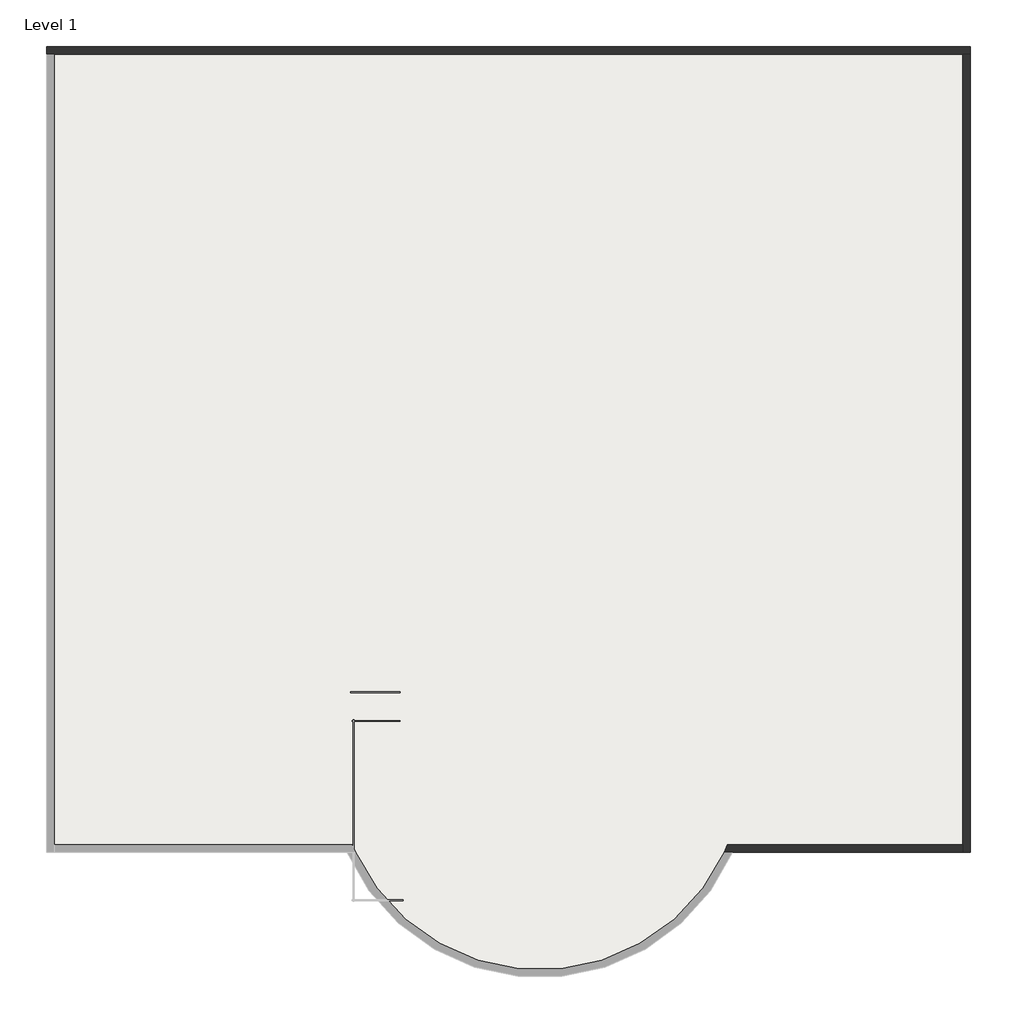
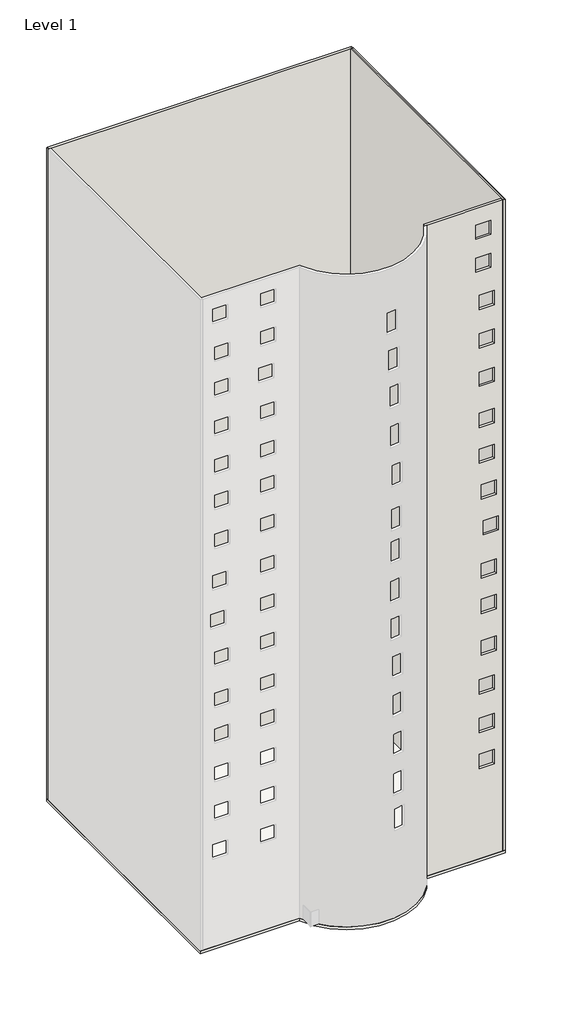
# One storey, part 3 of 3: 3 walls, 1 slab.
"""IFC4 building model written with IfcOpenShell, lengths in millimetres."""

from ifc_helpers import new_model, si_unit, point, frame, frame_2d, origin, place, context, project, spatial, polyline, circle_curve, trimmed, segment, composite_curve, outline, extrude, faceted_brep, element, save
from ifc_brep_helpers import plane_surface, revolved_surface, advanced_brep

model = new_model("IFC4")

# Units and contexts
model_context = context("Model", 3, world=origin())
ifc_project = project(units=[si_unit("LENGTHUNIT", "METRE", prefix="MILLI")], contexts=[model_context])

# Site, building, storey
site = spatial("IfcSite", under=ifc_project)
building = spatial("IfcBuilding", under=site)
storey = spatial("IfcBuildingStorey", under=building, Name="Level 1", Elevation=0.0)

# Slab
placement = place(None, origin())
element("IfcSlab", 1, ObjectType="9\"", at=placement, inside=storey, context=model_context, shape_type="SweptSolid", body=[
    extrude(outline(composite_curve([segment(polyline([(7979.2494573, 7359.5191779), (7979.2494573, -14078.0808221), (1652.8739931, -14078.0808221)]), True, "CONTINUOUS"), segment(trimmed(circle_curve(frame_2d((-3476.1505427, -11788.3650223)), 5616.9111737), [point((1652.8739931, -14078.0808221))], [point((-8605.1750786, -14078.0808221))], False, "CARTESIAN"), True, "CONTINUOUS"), segment(polyline([(-8605.1750786, -14078.0808221), (-16607.9505427, -14078.0808221), (-16607.9505427, 7359.5191779), (7979.2494573, 7359.5191779)]), True, "CONTINUOUS")], self_intersect=False)), frame((0.0, 0.0, -228.6), z_axis=(0.0, 0.0, 1.0), x_axis=(1.0, 0.0, 0.0)), (0.0, 0.0, 1.0), 228.6),
])

# Walls
element("IfcWall", 2, ObjectType="Generic - 8\"", at=placement, inside=storey, context=model_context, shape_type="Brep", body=[
    faceted_brep([(-16607.9505427, 7156.3191779, 0.0), (-16404.7505427, 7156.3191779, 0.0), (7776.0494573, 7156.3191779, 0.0), (7979.2494573, 7156.3191779, 0.0), (7979.2494573, 7156.3191779, 55473.6), (7928.4494573, 7156.3191779, 55473.6), (7776.0494573, 7156.3191779, 55473.6), (-16404.7505427, 7156.3191779, 55473.6), (-16556.2150607, 7156.3191779, 55473.6), (-16607.9505427, 7156.3191779, 55473.6), (-16607.9505427, 7359.5191779, 0.0), (-16607.9505427, 7359.5191779, 55473.6), (-16556.2150607, 7359.5191779, 55473.6), (7928.4494573, 7359.5191779, 55473.6), (7979.2494573, 7359.5191779, 55473.6), (7979.2494573, 7359.5191779, 0.0)], [[[0, 1, 2, 3, 4, 5, 6, 7, 8, 9]], [[10, 11, 12, 13, 14, 15]], [[3, 2, 1, 0, 10, 15]], [[4, 3, 15, 14]], [[0, 9, 11, 10]], [[5, 4, 14, 13]], [[9, 8, 12, 11]], [[8, 7, 6, 5, 13, 12]]]),
])
element("IfcWall", 3, ObjectType="Generic - 8\"", at=placement, inside=storey, context=model_context, shape_type="Brep", body=[
    faceted_brep([(7776.0494573, 7156.3191779, 0.0), (7776.0494573, -13874.8808221, 0.0), (7776.0494573, -14078.0808221, 0.0), (7776.0494573, -14078.0808221, 55473.6), (7776.0494573, -13874.8808221, 55473.6), (7776.0494573, 7156.3191779, 55473.6), (7979.2494573, 7156.3191779, 0.0), (7979.2494573, 7156.3191779, 55473.6), (7979.2494573, -14078.0808221, 55473.6), (7979.2494573, -14078.0808221, 0.0), (7928.4494573, 7156.3191779, 55473.6), (7928.4494573, -14078.0808221, 55473.6)], [[[0, 1, 2, 3, 4, 5]], [[6, 7, 8, 9]], [[2, 1, 0, 6, 9]], [[0, 5, 10, 7, 6]], [[3, 2, 9, 8, 11]], [[11, 8, 7, 10]], [[5, 4, 3, 11, 10]]]),
])
element("IfcWall", 4, ObjectType="Generic - 8\"", at=placement, inside=storey, context=model_context, shape_type="AdvancedBrep", body=[
    advanced_brep(
    [(7776.0494573, -13874.8808221, 0.0), (1519.3194541, -13874.8808221, 0.0), (1519.3194541, -13874.8808221, 55473.6), (7776.0494573, -13874.8808221, 55473.6), (5591.6494573, -13874.8808221, 54087.6218415), (5591.6494573, -13874.8808221, 52868.4218415), (6810.8494573, -13874.8808221, 52868.4218415), (6810.8494573, -13874.8808221, 54087.6218415), (5591.6494573, -13874.8808221, 51282.6), (5591.6494573, -13874.8808221, 50063.4), (6810.8494573, -13874.8808221, 50063.4), (6810.8494573, -13874.8808221, 51282.6), (5896.4494573, -13874.8808221, 48006.0), (5896.4494573, -13874.8808221, 46786.8), (7115.6494573, -13874.8808221, 46786.8), (7115.6494573, -13874.8808221, 48006.0), (5896.4494573, -13874.8808221, 44729.4), (5896.4494573, -13874.8808221, 43510.2), (7115.6494573, -13874.8808221, 43510.2), (7115.6494573, -13874.8808221, 44729.4), (5896.4494573, -13874.8808221, 41452.8), (5896.4494573, -13874.8808221, 40233.6), (7115.6494573, -13874.8808221, 40233.6), (7115.6494573, -13874.8808221, 41452.8), (5896.4494573, -13874.8808221, 37947.6), (5896.4494573, -13874.8808221, 36728.4), (7115.6494573, -13874.8808221, 36728.4), (7115.6494573, -13874.8808221, 37947.6), (5896.4494573, -13874.8808221, 34899.6), (5896.4494573, -13874.8808221, 33680.4), (7115.6494573, -13874.8808221, 33680.4), (7115.6494573, -13874.8808221, 34899.6), (6048.8494573, -13874.8808221, 31805.6549022), (6048.8494573, -13874.8808221, 30586.4549022), (7268.0494573, -13874.8808221, 30586.4549022), (7268.0494573, -13874.8808221, 31805.6549022), (6201.2494573, -13874.8808221, 28691.6136494), (6201.2494573, -13874.8808221, 27472.4136494), (7420.4494573, -13874.8808221, 27472.4136494), (7420.4494573, -13874.8808221, 28691.6136494), (6048.8494573, -13874.8808221, 25069.8), (6048.8494573, -13874.8808221, 23850.6), (7268.0494573, -13874.8808221, 23850.6), (7268.0494573, -13874.8808221, 25069.8), (6048.8494573, -13874.8808221, 22033.5127534), (6048.8494573, -13874.8808221, 20814.3127534), (7268.0494573, -13874.8808221, 20814.3127534), (7268.0494573, -13874.8808221, 22033.5127534), (6048.8494573, -13874.8808221, 18516.6), (6048.8494573, -13874.8808221, 17297.4), (7268.0494573, -13874.8808221, 17297.4), (7268.0494573, -13874.8808221, 18516.6), (5896.4494573, -13874.8808221, 15240.0), (5896.4494573, -13874.8808221, 14020.8), (7115.6494573, -13874.8808221, 14020.8), (7115.6494573, -13874.8808221, 15240.0), (5896.4494573, -13874.8808221, 11963.4), (5896.4494573, -13874.8808221, 10744.2), (7115.6494573, -13874.8808221, 10744.2), (7115.6494573, -13874.8808221, 11963.4), (5896.4494573, -13874.8808221, 8876.0183808), (5896.4494573, -13874.8808221, 7656.8183808), (7115.6494573, -13874.8808221, 7656.8183808), (7115.6494573, -13874.8808221, 8876.0183808), (7776.0494573, -14078.0808221, 0.0), (7776.0494573, -14078.0808221, 55473.6), (1652.8739931, -14078.0808221, 55473.6), (1429.5064192, -14078.0808221, 55473.6), (1429.5064192, -14078.0808221, 0.0), (1652.8739931, -14078.0808221, 0.0), (5591.6494573, -14078.0808221, 54087.6218415), (6810.8494573, -14078.0808221, 54087.6218415), (6810.8494573, -14078.0808221, 52868.4218415), (5591.6494573, -14078.0808221, 52868.4218415), (5591.6494573, -14078.0808221, 51282.6), (6810.8494573, -14078.0808221, 51282.6), (6810.8494573, -14078.0808221, 50063.4), (5591.6494573, -14078.0808221, 50063.4), (5896.4494573, -14078.0808221, 48006.0), (7115.6494573, -14078.0808221, 48006.0), (7115.6494573, -14078.0808221, 46786.8), (5896.4494573, -14078.0808221, 46786.8), (5896.4494573, -14078.0808221, 44729.4), (7115.6494573, -14078.0808221, 44729.4), (7115.6494573, -14078.0808221, 43510.2), (5896.4494573, -14078.0808221, 43510.2), (5896.4494573, -14078.0808221, 41452.8), (7115.6494573, -14078.0808221, 41452.8), (7115.6494573, -14078.0808221, 40233.6), (5896.4494573, -14078.0808221, 40233.6), (5896.4494573, -14078.0808221, 37947.6), (7115.6494573, -14078.0808221, 37947.6), (7115.6494573, -14078.0808221, 36728.4), (5896.4494573, -14078.0808221, 36728.4), (5896.4494573, -14078.0808221, 34899.6), (7115.6494573, -14078.0808221, 34899.6), (7115.6494573, -14078.0808221, 33680.4), (5896.4494573, -14078.0808221, 33680.4), (6048.8494573, -14078.0808221, 31805.6549022), (7268.0494573, -14078.0808221, 31805.6549022), (7268.0494573, -14078.0808221, 30586.4549022), (6048.8494573, -14078.0808221, 30586.4549022), (6201.2494573, -14078.0808221, 28691.6136494), (7420.4494573, -14078.0808221, 28691.6136494), (7420.4494573, -14078.0808221, 27472.4136494), (6201.2494573, -14078.0808221, 27472.4136494), (6048.8494573, -14078.0808221, 25069.8), (7268.0494573, -14078.0808221, 25069.8), (7268.0494573, -14078.0808221, 23850.6), (6048.8494573, -14078.0808221, 23850.6), (6048.8494573, -14078.0808221, 22033.5127534), (7268.0494573, -14078.0808221, 22033.5127534), (7268.0494573, -14078.0808221, 20814.3127534), (6048.8494573, -14078.0808221, 20814.3127534), (6048.8494573, -14078.0808221, 18516.6), (7268.0494573, -14078.0808221, 18516.6), (7268.0494573, -14078.0808221, 17297.4), (6048.8494573, -14078.0808221, 17297.4), (5896.4494573, -14078.0808221, 15240.0), (7115.6494573, -14078.0808221, 15240.0), (7115.6494573, -14078.0808221, 14020.8), (5896.4494573, -14078.0808221, 14020.8), (5896.4494573, -14078.0808221, 11963.4), (7115.6494573, -14078.0808221, 11963.4), (7115.6494573, -14078.0808221, 10744.2), (5896.4494573, -14078.0808221, 10744.2), (5896.4494573, -14078.0808221, 8876.0183808), (7115.6494573, -14078.0808221, 8876.0183808), (7115.6494573, -14078.0808221, 7656.8183808), (5896.4494573, -14078.0808221, 7656.8183808)],
    [
        (0, 1),
        (1, 2),
        (2, 3),
        (3, 0),
        (4, 5),
        (5, 6),
        (6, 7),
        (7, 4),
        (8, 9),
        (9, 10),
        (10, 11),
        (11, 8),
        (12, 13),
        (13, 14),
        (14, 15),
        (15, 12),
        (16, 17),
        (17, 18),
        (18, 19),
        (19, 16),
        (20, 21),
        (21, 22),
        (22, 23),
        (23, 20),
        (24, 25),
        (25, 26),
        (26, 27),
        (27, 24),
        (28, 29),
        (29, 30),
        (30, 31),
        (31, 28),
        (32, 33),
        (33, 34),
        (34, 35),
        (35, 32),
        (36, 37),
        (37, 38),
        (38, 39),
        (39, 36),
        (40, 41),
        (41, 42),
        (42, 43),
        (43, 40),
        (44, 45),
        (45, 46),
        (46, 47),
        (47, 44),
        (48, 49),
        (49, 50),
        (50, 51),
        (51, 48),
        (52, 53),
        (53, 54),
        (54, 55),
        (55, 52),
        (56, 57),
        (57, 58),
        (58, 59),
        (59, 56),
        (60, 61),
        (61, 62),
        (62, 63),
        (63, 60),
        (64, 65),
        (65, 66),
        (66, 67),
        (67, 68),
        (68, 69),
        (69, 64),
        (70, 71),
        (71, 72),
        (72, 73),
        (73, 70),
        (74, 75),
        (75, 76),
        (76, 77),
        (77, 74),
        (78, 79),
        (79, 80),
        (80, 81),
        (81, 78),
        (82, 83),
        (83, 84),
        (84, 85),
        (85, 82),
        (86, 87),
        (87, 88),
        (88, 89),
        (89, 86),
        (90, 91),
        (91, 92),
        (92, 93),
        (93, 90),
        (94, 95),
        (95, 96),
        (96, 97),
        (97, 94),
        (98, 99),
        (99, 100),
        (100, 101),
        (101, 98),
        (102, 103),
        (103, 104),
        (104, 105),
        (105, 102),
        (106, 107),
        (107, 108),
        (108, 109),
        (109, 106),
        (110, 111),
        (111, 112),
        (112, 113),
        (113, 110),
        (114, 115),
        (115, 116),
        (116, 117),
        (117, 114),
        (118, 119),
        (119, 120),
        (120, 121),
        (121, 118),
        (122, 123),
        (123, 124),
        (124, 125),
        (125, 122),
        (126, 127),
        (127, 128),
        (128, 129),
        (129, 126),
        (0, 64),
        (68, 1, circle_curve(frame((-3476.1505427, -11788.3650223, 0.0), z_axis=(0.0, 0.0, 1.0), x_axis=(1.0, 0.0, 0.0)), 5413.7111737)),
        (3, 65),
        (67, 2, circle_curve(frame((-3476.1505427, -11788.3650223, 55473.6), z_axis=(0.0, 0.0, 1.0), x_axis=(1.0, 0.0, 0.0)), 5413.7111737)),
        (4, 70),
        (73, 5),
        (72, 6),
        (71, 7),
        (8, 74),
        (77, 9),
        (76, 10),
        (75, 11),
        (12, 78),
        (81, 13),
        (80, 14),
        (79, 15),
        (16, 82),
        (85, 17),
        (84, 18),
        (83, 19),
        (20, 86),
        (89, 21),
        (88, 22),
        (87, 23),
        (24, 90),
        (93, 25),
        (92, 26),
        (91, 27),
        (28, 94),
        (97, 29),
        (96, 30),
        (95, 31),
        (32, 98),
        (101, 33),
        (100, 34),
        (99, 35),
        (36, 102),
        (105, 37),
        (104, 38),
        (103, 39),
        (40, 106),
        (109, 41),
        (108, 42),
        (107, 43),
        (44, 110),
        (113, 45),
        (112, 46),
        (111, 47),
        (48, 114),
        (117, 49),
        (116, 50),
        (115, 51),
        (52, 118),
        (121, 53),
        (120, 54),
        (119, 55),
        (56, 122),
        (125, 57),
        (124, 58),
        (123, 59),
        (60, 126),
        (129, 61),
        (128, 62),
        (127, 63),
    ],
    [
        plane_surface(frame((7877.6494573, -13874.8808221, 0.0), z_axis=(0.0, 1.0, 0.0), x_axis=(-1.0, 0.0, 0.0))),
        plane_surface(frame((7877.6494573, -14078.0808221, 0.0), z_axis=(0.0, -1.0, 0.0), x_axis=(1.0, 0.0, 0.0))),
        plane_surface(frame((7877.6494573, -13874.8808221, 0.0), z_axis=(0.0, 0.0, -1.0), x_axis=(0.0, -1.0, 0.0))),
        plane_surface(frame((7776.0494573, 7359.5191779, 0.0), z_axis=(1.0, 0.0, 0.0), x_axis=(0.0, -1.0, 0.0))),
        revolved_surface(polyline([(1937.5606309999994, -11788.3650223, 0.0), (1937.5606309999994, -11788.3650223, 55473.6)]), (-3476.1505427, -11788.3650223, 0.0), (0.0, 0.0, -1.0)),
        plane_surface(frame((5591.6494573, -13874.8808221, 54087.6218415), z_axis=(1.0, 0.0, 0.0), x_axis=(0.0, -1.0, 0.0))),
        plane_surface(frame((5591.6494573, -13874.8808221, 52868.4218415), z_axis=(0.0, 0.0, 1.0), x_axis=(0.0, -1.0, 0.0))),
        plane_surface(frame((6810.8494573, -13874.8808221, 52868.4218415), z_axis=(-1.0, 0.0, 0.0), x_axis=(0.0, -1.0, 0.0))),
        plane_surface(frame((6810.8494573, -13874.8808221, 54087.6218415), z_axis=(0.0, 0.0, -1.0), x_axis=(0.0, -1.0, 0.0))),
        plane_surface(frame((5591.6494573, -13874.8808221, 51282.6), z_axis=(1.0, 0.0, 0.0), x_axis=(0.0, -1.0, 0.0))),
        plane_surface(frame((5591.6494573, -13874.8808221, 50063.4), z_axis=(0.0, 0.0, 1.0), x_axis=(0.0, -1.0, 0.0))),
        plane_surface(frame((6810.8494573, -13874.8808221, 50063.4), z_axis=(-1.0, 0.0, 0.0), x_axis=(0.0, -1.0, 0.0))),
        plane_surface(frame((6810.8494573, -13874.8808221, 51282.6), z_axis=(0.0, 0.0, -1.0), x_axis=(0.0, -1.0, 0.0))),
        plane_surface(frame((5896.4494573, -13874.8808221, 48006.0), z_axis=(1.0, 0.0, 0.0), x_axis=(0.0, -1.0, 0.0))),
        plane_surface(frame((5896.4494573, -13874.8808221, 46786.8), z_axis=(0.0, 0.0, 1.0), x_axis=(0.0, -1.0, 0.0))),
        plane_surface(frame((7115.6494573, -13874.8808221, 46786.8), z_axis=(-1.0, 0.0, 0.0), x_axis=(0.0, -1.0, 0.0))),
        plane_surface(frame((7115.6494573, -13874.8808221, 48006.0), z_axis=(0.0, 0.0, -1.0), x_axis=(0.0, -1.0, 0.0))),
        plane_surface(frame((5896.4494573, -13874.8808221, 44729.4), z_axis=(1.0, 0.0, 0.0), x_axis=(0.0, -1.0, 0.0))),
        plane_surface(frame((5896.4494573, -13874.8808221, 43510.2), z_axis=(0.0, 0.0, 1.0), x_axis=(0.0, -1.0, 0.0))),
        plane_surface(frame((7115.6494573, -13874.8808221, 43510.2), z_axis=(-1.0, 0.0, 0.0), x_axis=(0.0, -1.0, 0.0))),
        plane_surface(frame((7115.6494573, -13874.8808221, 44729.4), z_axis=(0.0, 0.0, -1.0), x_axis=(0.0, -1.0, 0.0))),
        plane_surface(frame((5896.4494573, -13874.8808221, 41452.8), z_axis=(1.0, 0.0, 0.0), x_axis=(0.0, -1.0, 0.0))),
        plane_surface(frame((5896.4494573, -13874.8808221, 40233.6), z_axis=(0.0, 0.0, 1.0), x_axis=(0.0, -1.0, 0.0))),
        plane_surface(frame((7115.6494573, -13874.8808221, 40233.6), z_axis=(-1.0, 0.0, 0.0), x_axis=(0.0, -1.0, 0.0))),
        plane_surface(frame((7115.6494573, -13874.8808221, 41452.8), z_axis=(0.0, 0.0, -1.0), x_axis=(0.0, -1.0, 0.0))),
        plane_surface(frame((5896.4494573, -13874.8808221, 37947.6), z_axis=(1.0, 0.0, 0.0), x_axis=(0.0, -1.0, 0.0))),
        plane_surface(frame((5896.4494573, -13874.8808221, 36728.4), z_axis=(0.0, 0.0, 1.0), x_axis=(0.0, -1.0, 0.0))),
        plane_surface(frame((7115.6494573, -13874.8808221, 36728.4), z_axis=(-1.0, 0.0, 0.0), x_axis=(0.0, -1.0, 0.0))),
        plane_surface(frame((7115.6494573, -13874.8808221, 37947.6), z_axis=(0.0, 0.0, -1.0), x_axis=(0.0, -1.0, 0.0))),
        plane_surface(frame((5896.4494573, -13874.8808221, 34899.6), z_axis=(1.0, 0.0, 0.0), x_axis=(0.0, -1.0, 0.0))),
        plane_surface(frame((5896.4494573, -13874.8808221, 33680.4), z_axis=(0.0, 0.0, 1.0), x_axis=(0.0, -1.0, 0.0))),
        plane_surface(frame((7115.6494573, -13874.8808221, 33680.4), z_axis=(-1.0, 0.0, 0.0), x_axis=(0.0, -1.0, 0.0))),
        plane_surface(frame((7115.6494573, -13874.8808221, 34899.6), z_axis=(0.0, 0.0, -1.0), x_axis=(0.0, -1.0, 0.0))),
        plane_surface(frame((6048.8494573, -13874.8808221, 31805.6549022), z_axis=(1.0, 0.0, 0.0), x_axis=(0.0, -1.0, 0.0))),
        plane_surface(frame((6048.8494573, -13874.8808221, 30586.4549022), z_axis=(0.0, 0.0, 1.0), x_axis=(0.0, -1.0, 0.0))),
        plane_surface(frame((7268.0494573, -13874.8808221, 30586.4549022), z_axis=(-1.0, 0.0, 0.0), x_axis=(0.0, -1.0, 0.0))),
        plane_surface(frame((7268.0494573, -13874.8808221, 31805.6549022), z_axis=(0.0, 0.0, -1.0), x_axis=(0.0, -1.0, 0.0))),
        plane_surface(frame((6201.2494573, -13874.8808221, 28691.6136494), z_axis=(1.0, 0.0, 0.0), x_axis=(0.0, -1.0, 0.0))),
        plane_surface(frame((6201.2494573, -13874.8808221, 27472.4136494), z_axis=(0.0, 0.0, 1.0), x_axis=(0.0, -1.0, 0.0))),
        plane_surface(frame((7420.4494573, -13874.8808221, 27472.4136494), z_axis=(-1.0, 0.0, 0.0), x_axis=(0.0, -1.0, 0.0))),
        plane_surface(frame((7420.4494573, -13874.8808221, 28691.6136494), z_axis=(0.0, 0.0, -1.0), x_axis=(0.0, -1.0, 0.0))),
        plane_surface(frame((6048.8494573, -13874.8808221, 25069.8), z_axis=(1.0, 0.0, 0.0), x_axis=(0.0, -1.0, 0.0))),
        plane_surface(frame((6048.8494573, -13874.8808221, 23850.6), z_axis=(0.0, 0.0, 1.0), x_axis=(0.0, -1.0, 0.0))),
        plane_surface(frame((7268.0494573, -13874.8808221, 23850.6), z_axis=(-1.0, 0.0, 0.0), x_axis=(0.0, -1.0, 0.0))),
        plane_surface(frame((7268.0494573, -13874.8808221, 25069.8), z_axis=(0.0, 0.0, -1.0), x_axis=(0.0, -1.0, 0.0))),
        plane_surface(frame((6048.8494573, -13874.8808221, 22033.5127534), z_axis=(1.0, 0.0, 0.0), x_axis=(0.0, -1.0, 0.0))),
        plane_surface(frame((6048.8494573, -13874.8808221, 20814.3127534), z_axis=(0.0, 0.0, 1.0), x_axis=(0.0, -1.0, 0.0))),
        plane_surface(frame((7268.0494573, -13874.8808221, 20814.3127534), z_axis=(-1.0, 0.0, 0.0), x_axis=(0.0, -1.0, 0.0))),
        plane_surface(frame((7268.0494573, -13874.8808221, 22033.5127534), z_axis=(0.0, 0.0, -1.0), x_axis=(0.0, -1.0, 0.0))),
        plane_surface(frame((6048.8494573, -13874.8808221, 18516.6), z_axis=(1.0, 0.0, 0.0), x_axis=(0.0, -1.0, 0.0))),
        plane_surface(frame((6048.8494573, -13874.8808221, 17297.4), z_axis=(0.0, 0.0, 1.0), x_axis=(0.0, -1.0, 0.0))),
        plane_surface(frame((7268.0494573, -13874.8808221, 17297.4), z_axis=(-1.0, 0.0, 0.0), x_axis=(0.0, -1.0, 0.0))),
        plane_surface(frame((7268.0494573, -13874.8808221, 18516.6), z_axis=(0.0, 0.0, -1.0), x_axis=(0.0, -1.0, 0.0))),
        plane_surface(frame((5896.4494573, -13874.8808221, 15240.0), z_axis=(1.0, 0.0, 0.0), x_axis=(0.0, -1.0, 0.0))),
        plane_surface(frame((5896.4494573, -13874.8808221, 14020.8), z_axis=(0.0, 0.0, 1.0), x_axis=(0.0, -1.0, 0.0))),
        plane_surface(frame((7115.6494573, -13874.8808221, 14020.8), z_axis=(-1.0, 0.0, 0.0), x_axis=(0.0, -1.0, 0.0))),
        plane_surface(frame((7115.6494573, -13874.8808221, 15240.0), z_axis=(0.0, 0.0, -1.0), x_axis=(0.0, -1.0, 0.0))),
        plane_surface(frame((5896.4494573, -13874.8808221, 11963.4), z_axis=(1.0, 0.0, 0.0), x_axis=(0.0, -1.0, 0.0))),
        plane_surface(frame((5896.4494573, -13874.8808221, 10744.2), z_axis=(0.0, 0.0, 1.0), x_axis=(0.0, -1.0, 0.0))),
        plane_surface(frame((7115.6494573, -13874.8808221, 10744.2), z_axis=(-1.0, 0.0, 0.0), x_axis=(0.0, -1.0, 0.0))),
        plane_surface(frame((7115.6494573, -13874.8808221, 11963.4), z_axis=(0.0, 0.0, -1.0), x_axis=(0.0, -1.0, 0.0))),
        plane_surface(frame((5896.4494573, -13874.8808221, 8876.0183808), z_axis=(1.0, 0.0, 0.0), x_axis=(0.0, -1.0, 0.0))),
        plane_surface(frame((5896.4494573, -13874.8808221, 7656.8183808), z_axis=(0.0, 0.0, 1.0), x_axis=(0.0, -1.0, 0.0))),
        plane_surface(frame((7115.6494573, -13874.8808221, 7656.8183808), z_axis=(-1.0, 0.0, 0.0), x_axis=(0.0, -1.0, 0.0))),
        plane_surface(frame((7115.6494573, -13874.8808221, 8876.0183808), z_axis=(0.0, 0.0, -1.0), x_axis=(0.0, -1.0, 0.0))),
        plane_surface(frame((-16607.9505427, 7359.5191779, 55473.6), z_axis=(0.0, 0.0, 1.0), x_axis=(1.0, 0.0, 0.0))),
    ],
    [
        (0, [[1, 2, 3, 4], [5, 6, 7, 8], [9, 10, 11, 12], [13, 14, 15, 16], [17, 18, 19, 20], [21, 22, 23, 24], [25, 26, 27, 28], [29, 30, 31, 32], [33, 34, 35, 36], [37, 38, 39, 40], [41, 42, 43, 44], [45, 46, 47, 48], [49, 50, 51, 52], [53, 54, 55, 56], [57, 58, 59, 60], [61, 62, 63, 64]]),
        (1, [[65, 66, 67, 68, 69, 70], [71, 72, 73, 74], [75, 76, 77, 78], [79, 80, 81, 82], [83, 84, 85, 86], [87, 88, 89, 90], [91, 92, 93, 94], [95, 96, 97, 98], [99, 100, 101, 102], [103, 104, 105, 106], [107, 108, 109, 110], [111, 112, 113, 114], [115, 116, 117, 118], [119, 120, 121, 122], [123, 124, 125, 126], [127, 128, 129, 130]]),
        (2, [[-1, 131, -70, -69, 132]]),
        (3, [[-4, 133, -65, -131]]),
        (4, [[-2, -132, -68, 134]]),
        (5, [[-5, 135, -74, 136]]),
        (6, [[-6, -136, -73, 137]]),
        (7, [[-7, -137, -72, 138]]),
        (8, [[-8, -138, -71, -135]]),
        (9, [[-9, 139, -78, 140]]),
        (10, [[-10, -140, -77, 141]]),
        (11, [[-11, -141, -76, 142]]),
        (12, [[-12, -142, -75, -139]]),
        (13, [[-13, 143, -82, 144]]),
        (14, [[-14, -144, -81, 145]]),
        (15, [[-15, -145, -80, 146]]),
        (16, [[-16, -146, -79, -143]]),
        (17, [[-17, 147, -86, 148]]),
        (18, [[-18, -148, -85, 149]]),
        (19, [[-19, -149, -84, 150]]),
        (20, [[-20, -150, -83, -147]]),
        (21, [[-21, 151, -90, 152]]),
        (22, [[-22, -152, -89, 153]]),
        (23, [[-23, -153, -88, 154]]),
        (24, [[-24, -154, -87, -151]]),
        (25, [[-25, 155, -94, 156]]),
        (26, [[-26, -156, -93, 157]]),
        (27, [[-27, -157, -92, 158]]),
        (28, [[-28, -158, -91, -155]]),
        (29, [[-29, 159, -98, 160]]),
        (30, [[-30, -160, -97, 161]]),
        (31, [[-31, -161, -96, 162]]),
        (32, [[-32, -162, -95, -159]]),
        (33, [[-33, 163, -102, 164]]),
        (34, [[-34, -164, -101, 165]]),
        (35, [[-35, -165, -100, 166]]),
        (36, [[-36, -166, -99, -163]]),
        (37, [[-37, 167, -106, 168]]),
        (38, [[-38, -168, -105, 169]]),
        (39, [[-39, -169, -104, 170]]),
        (40, [[-40, -170, -103, -167]]),
        (41, [[-41, 171, -110, 172]]),
        (42, [[-42, -172, -109, 173]]),
        (43, [[-43, -173, -108, 174]]),
        (44, [[-44, -174, -107, -171]]),
        (45, [[-45, 175, -114, 176]]),
        (46, [[-46, -176, -113, 177]]),
        (47, [[-47, -177, -112, 178]]),
        (48, [[-48, -178, -111, -175]]),
        (49, [[-49, 179, -118, 180]]),
        (50, [[-50, -180, -117, 181]]),
        (51, [[-51, -181, -116, 182]]),
        (52, [[-52, -182, -115, -179]]),
        (53, [[-53, 183, -122, 184]]),
        (54, [[-54, -184, -121, 185]]),
        (55, [[-55, -185, -120, 186]]),
        (56, [[-56, -186, -119, -183]]),
        (57, [[-57, 187, -126, 188]]),
        (58, [[-58, -188, -125, 189]]),
        (59, [[-59, -189, -124, 190]]),
        (60, [[-60, -190, -123, -187]]),
        (61, [[-61, 191, -130, 192]]),
        (62, [[-62, -192, -129, 193]]),
        (63, [[-63, -193, -128, 194]]),
        (64, [[-64, -194, -127, -191]]),
        (65, [[-3, -134, -67, -66, -133]]),
    ],
),
])

save(model, "model.ifc")

# Revit data of these elements
# Type "9\""
#   Assembly Code = "B1010"
#   Function = 0
#   Layers, outside or top first: 0' - 9" no material (function 1)
# Type "Generic - 8\""
#   Assembly Code = "B2010"
#   Layers, outside or top first: 0' - 8" no material (function 1)
# Element 1 (IfcSlab, "9\"")
#   Height Offset From Level = 0' - 0"
#   Phase Created = New Construction
#   Materials on its faces: "Default Floor"
# Elements 2, 3, 4 (IfcWall, "Generic - 8\"")
#   Top Offset = 0' - 0"
#   Base Offset = 0' - 0"
#   Unconnected Height = 182' - 0"
#   wall height = 182' - 0"
#   Phase Created = New Construction
#   Base Constraint = Level 1
#   Materials on its faces: "Default Wall"
# Materials
#   "Default Floor": colour RGB 128 128 128, transparency 0
#   "Default Wall": colour RGB 128 128 128, transparency 0
